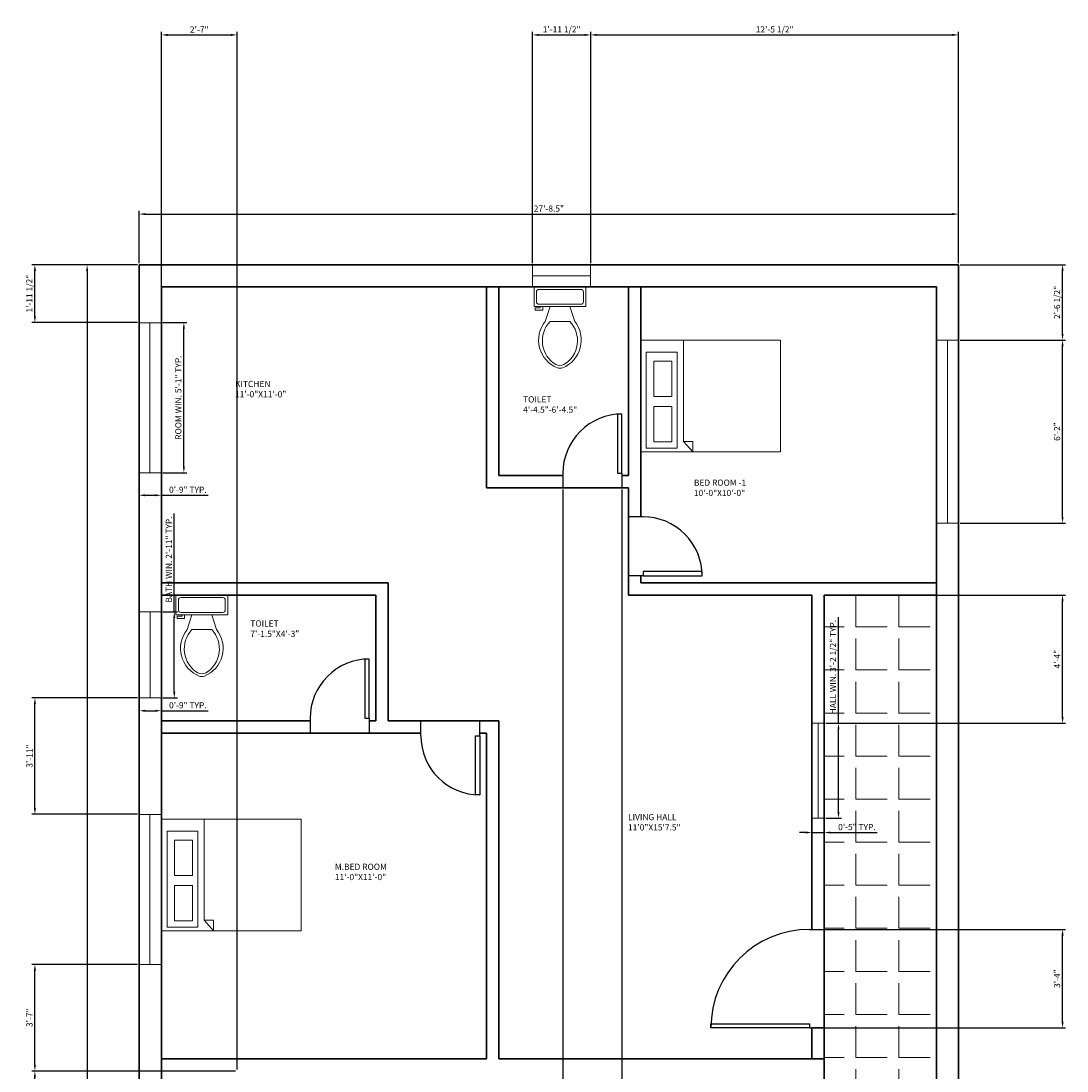
# Model space of a CAD drawing. Units: inches. Extents: x 4673 to 5097, y 7020 to 7947.
# Tile 3 of 3: x 4673 to 5097, y 7521 to 7947. Entities that reach past the tile are written whole.
import ezdxf

# ---------------------------------------------------------------- set-up
doc = ezdxf.new("R2010")
doc.units = ezdxf.units.IN
for name, color, linetype, lineweight in [('A-ANNO-DIMS', 244, 'Continuous', 18), ('A-AREA-IDEN', 7, 'Continuous', 18), ('A-DOOR', 4, 'Continuous', 25), ('A-FLOR-FIXT', 8, 'Continuous', 18), ('A-FLOR-PATT', 9, 'Continuous', 13), ('A-FURN', 152, 'Continuous', 18), ('A-GLAZ', 152, 'Continuous', 18), ('A-WALL', 7, 'Continuous', 35)]:
    doc.layers.add(name, color=color, linetype=linetype, lineweight=lineweight)
doc.styles.get("Standard").update_dxf_attribs({"font": 'arial.ttf'})
doc.dimstyles.new('ISO-25', dxfattribs={"dimtxt": 2.5, "dimasz": 2.5, "dimexe": 1.25, "dimexo": 0.625, "dimtad": 1, "dimlunit": 3, "dimtxsty": 'Standard', "dimcen": 2.5, "dimadec": 0, "dimazin": 0, "dimtfac": 1, "dimtmove": 0, "dimatfit": 3, "dimfxl": 1, "dimarcsym": 0})

# ---------------------------------------------------------------- blocks, each defined once
blk = doc.blocks.new('*U5')
for p, q in [((0, 0), (0, 6)), ((24, 0), (24, 6))]:
    blk.add_line(p, q)
blk.add_lwpolyline([(0, 0), (0, -24), (1.75, -24), (1.75, 0)], close=True)
blk.add_arc((0, 0), 24, 270, 0)
blk = doc.blocks.new('*U3')
for p, q in [((0, 0), (0, -6)), ((40, 0), (40, -6))]:
    blk.add_line(p, q)
blk.add_lwpolyline([(0, 0), (0, 40), (1.75, 40), (1.75, 0)], close=True)
blk.add_arc((0, 0), 40, 0, 90)
blk = doc.blocks.new('*U4')
for p, q in [((0, 0), (0, -6)), ((24, 0), (24, -6))]:
    blk.add_line(p, q)
blk.add_lwpolyline([(0, 0), (0, 24), (1.75, 24), (1.75, 0)], close=True)
blk.add_arc((0, 0), 24, 0, 90)
blk = doc.blocks.new('*U8')
for p, q in [((9.5, -6), (9.5, -2)), ((-10, -8.5), (-8, -8.5)), ((-10, -9.5), (-10, -8.5)), ((-8, -8.5), (-8, -8)), ((-7, -8), (-7, -9.5)), ((-4, -8), (-6, -14)), ((4, -8), (6, -14)), ((-7, -9.5), (-10, -9.5)), ((4, -14), (-4, -14))]:
    blk.add_line(p, q)
blk.add_lwpolyline([(10.5, -8), (10.5, 0), (-10.5, 0), (-10.5, -8)], close=True)
for points in [[(-9.5, -2), (-9.5, -6)], [(8.5, -1), (-8.5, -1)], [(-8.5, -7), (8.5, -7)]]:
    blk.add_lwpolyline(points)
for centre, radius, start, end in [((-8.62, -1.88), 0.884, 81.8699, 188.1301), ((8.62, -1.88), 0.884, 351.8699, 98.1301), ((-8.62, -6.12), 0.884, 171.8699, 278.1301), ((8.62, -6.12), 0.884, 261.8699, 8.1301), ((3.52, -21.58), 12.17, 141.4691, 247.9714), ((4.2, -21.82), 11.33, 136.3677, 238.9468), ((-3.52, -21.58), 12.17, 292.0284, 38.5307), ((-4.2, -21.82), 11.33, 301.053, 43.6321), ((0, -27.88), 4, 245.7318, 294.2682), ((0, -29), 4, 254.8605, 285.1395)]:
    blk.add_arc(centre, radius, start, end)
blk = doc.blocks.new('*D9')
at = {"layer": 'A-ANNO-DIMS', "color": 0, "lineweight": -2, "transparency": 16777216}
for p, q in [((4720.89, 7848.49), (4720.89, 7869.66)), ((4723.39, 7868.41), (5050.89, 7868.41)), ((5053.39, 7848.49), (5053.39, 7869.66))]:
    blk.add_line(p, q, dxfattribs=at)
at = {"layer": 'A-ANNO-DIMS', "color": 0, "transparency": 16777216}
for points in [[(4723.39, 7868.83), (4723.39, 7868), (4720.89, 7868.41)], [(5050.89, 7868.83), (5050.89, 7868), (5053.39, 7868.41)]]:
    blk.add_solid(points, dxfattribs=at)
at = {"layer": 'Defpoints', "color": 0, "transparency": 16777216}
for p in [(5053.39, 7868.41), (4720.89, 7847.86), (5053.39, 7847.86)]:
    blk.add_point(p, dxfattribs=at)
at = {"layer": 'A-ANNO-DIMS', "color": 0, "transparency": 16777216, "insert": (4887.14, 7870.32), "char_height": 2.5, "attachment_point": 5}
blk.add_mtext('27\'-8.5"', dxfattribs=at)
blk = doc.blocks.new('*D10')
at = {"layer": 'A-ANNO-DIMS', "color": 0, "lineweight": -2, "transparency": 16777216}
for p, q in [((4720.26, 7847.86), (4698.51, 7847.86)), ((4699.76, 7845.36), (4699.76, 7117.36)), ((4720.26, 7114.86), (4698.51, 7114.86))]:
    blk.add_line(p, q, dxfattribs=at)
at = {"layer": 'A-ANNO-DIMS', "color": 0, "transparency": 16777216}
for points in [[(4699.34, 7845.36), (4700.18, 7845.36), (4699.76, 7847.86)], [(4699.34, 7117.36), (4700.18, 7117.36), (4699.76, 7114.86)]]:
    blk.add_solid(points, dxfattribs=at)
at = {"layer": 'Defpoints', "color": 0, "transparency": 16777216}
for p in [(4720.89, 7847.86), (4699.76, 7114.86), (4720.89, 7114.86)]:
    blk.add_point(p, dxfattribs=at)
at = {"layer": 'A-ANNO-DIMS', "color": 0, "transparency": 16777216, "insert": (4697.86, 7481.36), "char_height": 2.5, "attachment_point": 5, "rotation": 90}
blk.add_mtext('61\'-1"', dxfattribs=at)
blk = doc.blocks.new('BED-DOUBLE')
for p, q in [((17.35, 45.28), (17.35, 4.23)), ((17.35, 4.23), (21.14, 0)), ((17.35, 4.23), (21.14, 4.23)), ((21.14, 0), (21.14, 4.23))]:
    blk.add_line(p, q)
for points in [[(0, 0), (0, 45.28), (56.77, 45.28), (56.77, 0)], [(2.29, 1.5), (2.29, 40.39), (14.79, 40.39), (14.79, 1.5)], [(5.28, 22.37), (5.28, 36.69), (12.64, 36.69), (12.64, 22.37)], [(5.28, 4.03), (5.28, 18.35), (12.64, 18.35), (12.64, 4.03)]]:
    blk.add_lwpolyline(points, close=True)
blk = doc.blocks.new('WIN-61IN')
for p, q in [((9, 60.82), (0, 60.82)), ((0.12, 60.89), (0.12, 0.07)), ((9, 60.82), (4.5, 60.82)), ((4.5, 60.82), (4.5, 0)), ((9.12, 0), (9.12, 60.82)), ((0, 0), (9, 0))]:
    blk.add_line(p, q)
blk = doc.blocks.new('WIN-HALL-38IN')
for p, q in [((5, 38.52), (0, 38.52)), ((0, 38.52), (0, 0)), ((5, 38.52), (2.5, 38.52)), ((2.5, 38.52), (2.5, 0)), ((5, 0), (5, 38.52)), ((0, 0), (5, 0))]:
    blk.add_line(p, q)
blk = doc.blocks.new('WIN-BATH-35IN')
for p, q in [((9, 34.94), (0, 34.94)), ((0, 34.94), (0, 0)), ((9, 34.94), (4.5, 34.94)), ((4.5, 34.94), (4.5, 0)), ((9, 0), (9, 34.94)), ((0, 0), (9, 0))]:
    blk.add_line(p, q)
blk = doc.blocks.new('*D17')
at = {"layer": 'A-ANNO-DIMS', "color": 0, "lineweight": -2, "transparency": 16777216}
for p, q in [((4730.51, 7824.39), (4740.27, 7824.39)), ((4739.02, 7766), (4739.02, 7821.89)), ((4730.51, 7763.5), (4740.27, 7763.5))]:
    blk.add_line(p, q, dxfattribs=at)
at = {"layer": 'A-ANNO-DIMS', "color": 0, "transparency": 16777216}
for points in [[(4738.6, 7821.89), (4739.44, 7821.89), (4739.02, 7824.39)], [(4738.6, 7766), (4739.44, 7766), (4739.02, 7763.5)]]:
    blk.add_solid(points, dxfattribs=at)
at = {"layer": 'Defpoints', "color": 0, "transparency": 16777216}
for p in [(4729.89, 7824.39), (4739.02, 7824.39), (4729.89, 7763.5)]:
    blk.add_point(p, dxfattribs=at)
at = {"layer": 'A-ANNO-DIMS', "color": 0, "transparency": 16777216, "insert": (4737.1, 7793.94), "char_height": 2.5, "attachment_point": 5, "rotation": 90}
blk.add_mtext('ROOM WIN. 5\'-1" TYP.', dxfattribs=at)
blk = doc.blocks.new('*D18')
at = {"layer": 'A-ANNO-DIMS', "color": 0, "lineweight": -2, "transparency": 16777216}
for p, q in [((4720.77, 7762.88), (4720.77, 7753.12)), ((4729.89, 7762.88), (4729.89, 7753.12)), ((4723.27, 7754.37), (4727.39, 7754.37)), ((4729.89, 7754.37), (4748.88, 7754.37))]:
    blk.add_line(p, q, dxfattribs=at)
at = {"layer": 'A-ANNO-DIMS', "color": 0, "transparency": 16777216}
for points in [[(4723.27, 7754.78), (4723.27, 7753.95), (4720.77, 7754.37)], [(4727.39, 7754.78), (4727.39, 7753.95), (4729.89, 7754.37)]]:
    blk.add_solid(points, dxfattribs=at)
at = {"layer": 'Defpoints', "color": 0, "transparency": 16777216}
for p in [(4720.77, 7763.5), (4729.89, 7763.5), (4729.89, 7754.37)]:
    blk.add_point(p, dxfattribs=at)
at = {"layer": 'A-ANNO-DIMS', "color": 0, "transparency": 16777216, "insert": (4740.63, 7756.27), "char_height": 2.5, "attachment_point": 5}
blk.add_mtext('0\'-9" TYP.', dxfattribs=at)
blk = doc.blocks.new('*D19')
at = {"layer": 'A-ANNO-DIMS', "color": 0, "lineweight": -2, "transparency": 16777216}
for p, q in [((4735.13, 7707.15), (4735.13, 7746.98)), ((4730.51, 7707.15), (4736.38, 7707.15)), ((4735.13, 7674.7), (4735.13, 7704.65)), ((4730.51, 7672.2), (4736.38, 7672.2))]:
    blk.add_line(p, q, dxfattribs=at)
at = {"layer": 'A-ANNO-DIMS', "color": 0, "transparency": 16777216}
for points in [[(4734.71, 7704.65), (4735.55, 7704.65), (4735.13, 7707.15)], [(4734.71, 7674.7), (4735.55, 7674.7), (4735.13, 7672.2)]]:
    blk.add_solid(points, dxfattribs=at)
at = {"layer": 'Defpoints', "color": 0, "transparency": 16777216}
for p in [(4729.89, 7707.15), (4735.13, 7707.15), (4729.89, 7672.2)]:
    blk.add_point(p, dxfattribs=at)
at = {"layer": 'A-ANNO-DIMS', "color": 0, "transparency": 16777216, "insert": (4733.25, 7728.31), "char_height": 2.5, "attachment_point": 5, "rotation": 90}
blk.add_mtext('BATH WIN. 2\'-11" TYP.', dxfattribs=at)
blk = doc.blocks.new('*D20')
at = {"layer": 'A-ANNO-DIMS', "color": 0, "lineweight": -2, "transparency": 16777216}
for p, q in [((4720.89, 7671.58), (4720.89, 7665.71)), ((4729.89, 7671.58), (4729.89, 7665.71)), ((4723.39, 7666.96), (4727.39, 7666.96)), ((4729.89, 7666.96), (4748.88, 7666.96))]:
    blk.add_line(p, q, dxfattribs=at)
at = {"layer": 'A-ANNO-DIMS', "color": 0, "transparency": 16777216}
for points in [[(4723.39, 7667.38), (4723.39, 7666.54), (4720.89, 7666.96)], [(4727.39, 7667.38), (4727.39, 7666.54), (4729.89, 7666.96)]]:
    blk.add_solid(points, dxfattribs=at)
at = {"layer": 'Defpoints', "color": 0, "transparency": 16777216}
for p in [(4720.89, 7672.2), (4729.89, 7672.2), (4729.89, 7666.96)]:
    blk.add_point(p, dxfattribs=at)
at = {"layer": 'A-ANNO-DIMS', "color": 0, "transparency": 16777216, "insert": (4740.63, 7668.86), "char_height": 2.5, "attachment_point": 5}
blk.add_mtext('0\'-9" TYP.', dxfattribs=at)
blk = doc.blocks.new('*D21')
at = {"layer": 'A-ANNO-DIMS', "color": 0, "lineweight": -2, "transparency": 16777216}
for p, q in [((5004.67, 7661.88), (5004.67, 7704.99)), ((4999.51, 7661.88), (5005.92, 7661.88)), ((5004.67, 7625.86), (5004.67, 7659.38)), ((4999.51, 7623.36), (5005.92, 7623.36))]:
    blk.add_line(p, q, dxfattribs=at)
at = {"layer": 'A-ANNO-DIMS', "color": 0, "transparency": 16777216}
for points in [[(5004.25, 7659.38), (5005.08, 7659.38), (5004.67, 7661.88)], [(5004.25, 7625.86), (5005.08, 7625.86), (5004.67, 7623.36)]]:
    blk.add_solid(points, dxfattribs=at)
at = {"layer": 'Defpoints', "color": 0, "transparency": 16777216}
for p in [(4998.89, 7661.88), (5004.67, 7661.88), (4998.89, 7623.36)]:
    blk.add_point(p, dxfattribs=at)
at = {"layer": 'A-ANNO-DIMS', "color": 0, "transparency": 16777216, "insert": (5002.75, 7684.68), "char_height": 2.5, "attachment_point": 5, "rotation": 90}
blk.add_mtext('HALL WIN. 3\'-2 1/2" TYP.', dxfattribs=at)
blk = doc.blocks.new('*D22')
at = {"layer": 'A-ANNO-DIMS', "color": 0, "lineweight": -2, "transparency": 16777216}
for p, q in [((4993.89, 7622.73), (4993.89, 7616.33)), ((4998.89, 7622.73), (4998.89, 7616.33)), ((4991.39, 7617.58), (4988.89, 7617.58)), ((4993.89, 7617.58), (4998.89, 7617.58)), ((5001.39, 7617.58), (5020.38, 7617.58))]:
    blk.add_line(p, q, dxfattribs=at)
at = {"layer": 'A-ANNO-DIMS', "color": 0, "transparency": 16777216}
for points in [[(4991.39, 7617.99), (4991.39, 7617.16), (4993.89, 7617.58)], [(5001.39, 7617.99), (5001.39, 7617.16), (4998.89, 7617.58)]]:
    blk.add_solid(points, dxfattribs=at)
at = {"layer": 'Defpoints', "color": 0, "transparency": 16777216}
for p in [(4993.89, 7623.36), (4998.89, 7623.36), (4998.89, 7617.58)]:
    blk.add_point(p, dxfattribs=at)
at = {"layer": 'A-ANNO-DIMS', "color": 0, "transparency": 16777216, "insert": (5012.13, 7619.48), "char_height": 2.5, "attachment_point": 5}
blk.add_mtext('0\'-5" TYP.', dxfattribs=at)
blk = doc.blocks.new('*D25')
at = {"layer": 'A-ANNO-DIMS', "color": 0, "lineweight": -2, "transparency": 16777216}
for p, q in [((5054.01, 7817.28), (5096.84, 7817.28)), ((5095.59, 7745.59), (5095.59, 7814.78)), ((5054.01, 7743.09), (5096.84, 7743.09))]:
    blk.add_line(p, q, dxfattribs=at)
at = {"layer": 'A-ANNO-DIMS', "color": 0, "transparency": 16777216}
for points in [[(5095.17, 7814.78), (5096.01, 7814.78), (5095.59, 7817.28)], [(5095.17, 7745.59), (5096.01, 7745.59), (5095.59, 7743.09)]]:
    blk.add_solid(points, dxfattribs=at)
at = {"layer": 'Defpoints', "color": 0, "transparency": 16777216}
for p in [(5053.39, 7817.28), (5095.59, 7817.28), (5053.39, 7743.09)]:
    blk.add_point(p, dxfattribs=at)
at = {"layer": 'A-ANNO-DIMS', "color": 0, "transparency": 16777216, "insert": (5093.69, 7780.18), "char_height": 2.5, "attachment_point": 5, "rotation": 90}
blk.add_mtext('6\'-2"', dxfattribs=at)
blk = doc.blocks.new('*D26')
at = {"layer": 'A-ANNO-DIMS', "color": 0, "lineweight": -2, "transparency": 16777216}
for p, q in [((5054.01, 7847.86), (5096.84, 7847.86)), ((5095.59, 7819.78), (5095.59, 7845.36)), ((5054.01, 7817.28), (5096.84, 7817.28))]:
    blk.add_line(p, q, dxfattribs=at)
at = {"layer": 'A-ANNO-DIMS', "color": 0, "transparency": 16777216}
for points in [[(5095.17, 7845.36), (5096.01, 7845.36), (5095.59, 7847.86)], [(5095.17, 7819.78), (5096.01, 7819.78), (5095.59, 7817.28)]]:
    blk.add_solid(points, dxfattribs=at)
at = {"layer": 'Defpoints', "color": 0, "transparency": 16777216}
for p in [(5053.39, 7847.86), (5095.59, 7847.86), (5053.39, 7817.28)]:
    blk.add_point(p, dxfattribs=at)
at = {"layer": 'A-ANNO-DIMS', "color": 0, "transparency": 16777216, "insert": (5093.67, 7832.57), "char_height": 2.5, "attachment_point": 5, "rotation": 90}
blk.add_mtext('2\'-6 1/2"', dxfattribs=at)
blk = doc.blocks.new('*D27')
at = {"layer": 'A-ANNO-DIMS', "color": 0, "lineweight": -2, "transparency": 16777216}
for p, q in [((4880.5, 7848.49), (4880.5, 7942.32)), ((4904.1, 7848.49), (4904.1, 7942.32)), ((4883, 7941.07), (4901.6, 7941.07))]:
    blk.add_line(p, q, dxfattribs=at)
at = {"layer": 'A-ANNO-DIMS', "color": 0, "transparency": 16777216}
for points in [[(4883, 7941.49), (4883, 7940.65), (4880.5, 7941.07)], [(4901.6, 7941.49), (4901.6, 7940.65), (4904.1, 7941.07)]]:
    blk.add_solid(points, dxfattribs=at)
at = {"layer": 'Defpoints', "color": 0, "transparency": 16777216}
for p in [(4904.1, 7941.07), (4880.5, 7847.86), (4904.1, 7847.86)]:
    blk.add_point(p, dxfattribs=at)
at = {"layer": 'A-ANNO-DIMS', "color": 0, "transparency": 16777216, "insert": (4892.3, 7942.99), "char_height": 2.5, "attachment_point": 5}
blk.add_mtext('1\'-11 1/2"', dxfattribs=at)
blk = doc.blocks.new('*D28')
at = {"layer": 'A-ANNO-DIMS', "color": 0, "lineweight": -2, "transparency": 16777216}
for p, q in [((4904.1, 7848.49), (4904.1, 7942.32)), ((5053.39, 7848.49), (5053.39, 7942.32)), ((4906.6, 7941.07), (5050.89, 7941.07))]:
    blk.add_line(p, q, dxfattribs=at)
at = {"layer": 'A-ANNO-DIMS', "color": 0, "transparency": 16777216}
for points in [[(4906.6, 7941.49), (4906.6, 7940.65), (4904.1, 7941.07)], [(5050.89, 7941.49), (5050.89, 7940.65), (5053.39, 7941.07)]]:
    blk.add_solid(points, dxfattribs=at)
at = {"layer": 'Defpoints', "color": 0, "transparency": 16777216}
for p in [(5053.39, 7941.07), (4904.1, 7847.86), (5053.39, 7847.86)]:
    blk.add_point(p, dxfattribs=at)
at = {"layer": 'A-ANNO-DIMS', "color": 0, "transparency": 16777216, "insert": (4978.74, 7942.99), "char_height": 2.5, "attachment_point": 5}
blk.add_mtext('12\'-5 1/2"', dxfattribs=at)
blk = doc.blocks.new('*D31')
at = {"layer": 'A-ANNO-DIMS', "color": 0, "lineweight": -2, "transparency": 16777216}
for p, q in [((4729.89, 7521.49), (4729.89, 7942.32)), ((4760.64, 7521.49), (4760.64, 7942.32)), ((4732.39, 7941.07), (4758.14, 7941.07))]:
    blk.add_line(p, q, dxfattribs=at)
at = {"layer": 'A-ANNO-DIMS', "color": 0, "transparency": 16777216}
for points in [[(4732.39, 7941.49), (4732.39, 7940.65), (4729.89, 7941.07)], [(4758.14, 7941.49), (4758.14, 7940.65), (4760.64, 7941.07)]]:
    blk.add_solid(points, dxfattribs=at)
at = {"layer": 'Defpoints', "color": 0, "transparency": 16777216}
for p in [(4760.64, 7941.07), (4729.89, 7520.86), (4760.64, 7520.86)]:
    blk.add_point(p, dxfattribs=at)
at = {"layer": 'A-ANNO-DIMS', "color": 0, "transparency": 16777216, "insert": (4745.26, 7942.95), "char_height": 2.5, "attachment_point": 5}
blk.add_mtext('2\'-7"', dxfattribs=at)
blk = doc.blocks.new('*D32')
at = {"layer": 'A-ANNO-DIMS', "color": 0, "lineweight": -2, "transparency": 16777216}
for p, q in [((4760.01, 7520.86), (4677.32, 7520.86)), ((4678.57, 7493.36), (4678.57, 7518.36)), ((4760.01, 7490.86), (4677.32, 7490.86))]:
    blk.add_line(p, q, dxfattribs=at)
at = {"layer": 'A-ANNO-DIMS', "color": 0, "transparency": 16777216}
for points in [[(4678.15, 7518.36), (4678.99, 7518.36), (4678.57, 7520.86)], [(4678.15, 7493.36), (4678.99, 7493.36), (4678.57, 7490.86)]]:
    blk.add_solid(points, dxfattribs=at)
at = {"layer": 'Defpoints', "color": 0, "transparency": 16777216}
for p in [(4678.57, 7520.86), (4760.64, 7520.86), (4760.64, 7490.86)]:
    blk.add_point(p, dxfattribs=at)
at = {"layer": 'A-ANNO-DIMS', "color": 0, "transparency": 16777216, "insert": (4676.67, 7505.86), "char_height": 2.5, "attachment_point": 5, "rotation": 90}
blk.add_mtext('2\'-6"', dxfattribs=at)
blk = doc.blocks.new('*D34')
at = {"layer": 'A-ANNO-DIMS', "color": 0, "lineweight": -2, "transparency": 16777216}
for p, q in [((4994.51, 7578.31), (5096.84, 7578.31)), ((5095.59, 7540.82), (5095.59, 7575.81)), ((4994.51, 7538.32), (5096.84, 7538.32))]:
    blk.add_line(p, q, dxfattribs=at)
at = {"layer": 'A-ANNO-DIMS', "color": 0, "transparency": 16777216}
for points in [[(5095.17, 7575.81), (5096.01, 7575.81), (5095.59, 7578.31)], [(5095.17, 7540.82), (5096.01, 7540.82), (5095.59, 7538.32)]]:
    blk.add_solid(points, dxfattribs=at)
at = {"layer": 'Defpoints', "color": 0, "transparency": 16777216}
for p in [(4993.89, 7578.31), (5095.59, 7578.31), (4993.89, 7538.32)]:
    blk.add_point(p, dxfattribs=at)
at = {"layer": 'A-ANNO-DIMS', "color": 0, "transparency": 16777216, "insert": (5093.69, 7558.31), "char_height": 2.5, "attachment_point": 5, "rotation": 90}
blk.add_mtext('3\'-4"', dxfattribs=at)
blk = doc.blocks.new('*D35')
at = {"layer": 'A-ANNO-DIMS', "color": 0, "lineweight": -2, "transparency": 16777216}
for p, q in [((4892.8, 7756.68), (4892.8, 7020.41)), ((4916.8, 7756.68), (4916.8, 7020.41)), ((4895.3, 7021.66), (4914.3, 7021.66))]:
    blk.add_line(p, q, dxfattribs=at)
at = {"layer": 'A-ANNO-DIMS', "color": 0, "transparency": 16777216}
for points in [[(4895.3, 7022.08), (4895.3, 7021.25), (4892.8, 7021.66)], [(4914.3, 7022.08), (4914.3, 7021.25), (4916.8, 7021.66)]]:
    blk.add_solid(points, dxfattribs=at)
at = {"layer": 'Defpoints', "color": 0, "transparency": 16777216}
for p in [(4892.8, 7757.31), (4916.8, 7757.31), (4916.8, 7021.66)]:
    blk.add_point(p, dxfattribs=at)
at = {"layer": 'A-ANNO-DIMS', "color": 0, "transparency": 16777216, "insert": (4904.8, 7023.56), "char_height": 2.5, "attachment_point": 5}
blk.add_mtext('2\'-0"', dxfattribs=at)
blk = doc.blocks.new('*D40')
at = {"layer": 'A-ANNO-DIMS', "color": 0, "lineweight": -2, "transparency": 16777216}
for p, q in [((4720.14, 7564.08), (4677.32, 7564.08)), ((4678.57, 7523.36), (4678.57, 7561.58)), ((4729.26, 7520.86), (4677.32, 7520.86))]:
    blk.add_line(p, q, dxfattribs=at)
at = {"layer": 'A-ANNO-DIMS', "color": 0, "transparency": 16777216}
for points in [[(4678.15, 7561.58), (4678.99, 7561.58), (4678.57, 7564.08)], [(4678.15, 7523.36), (4678.99, 7523.36), (4678.57, 7520.86)]]:
    blk.add_solid(points, dxfattribs=at)
at = {"layer": 'Defpoints', "color": 0, "transparency": 16777216}
for p in [(4678.57, 7564.08), (4720.77, 7564.08), (4729.89, 7520.86)]:
    blk.add_point(p, dxfattribs=at)
at = {"layer": 'A-ANNO-DIMS', "color": 0, "transparency": 16777216, "insert": (4676.67, 7542.47), "char_height": 2.5, "attachment_point": 5, "rotation": 90}
blk.add_mtext('3\'-7"', dxfattribs=at)
blk = doc.blocks.new('*D41')
at = {"layer": 'A-ANNO-DIMS', "color": 0, "lineweight": -2, "transparency": 16777216}
for p, q in [((4720.26, 7672.2), (4677.32, 7672.2)), ((4678.57, 7627.47), (4678.57, 7669.7)), ((4720.26, 7624.97), (4677.32, 7624.97))]:
    blk.add_line(p, q, dxfattribs=at)
at = {"layer": 'A-ANNO-DIMS', "color": 0, "transparency": 16777216}
for points in [[(4678.15, 7669.7), (4678.99, 7669.7), (4678.57, 7672.2)], [(4678.15, 7627.47), (4678.99, 7627.47), (4678.57, 7624.97)]]:
    blk.add_solid(points, dxfattribs=at)
at = {"layer": 'Defpoints', "color": 0, "transparency": 16777216}
for p in [(4678.57, 7672.2), (4720.89, 7672.2), (4720.89, 7624.97)]:
    blk.add_point(p, dxfattribs=at)
at = {"layer": 'A-ANNO-DIMS', "color": 0, "transparency": 16777216, "insert": (4676.67, 7648.59), "char_height": 2.5, "attachment_point": 5, "rotation": 90}
blk.add_mtext('3\'-11"', dxfattribs=at)
blk = doc.blocks.new('*D42')
at = {"layer": 'A-ANNO-DIMS', "color": 0, "lineweight": -2, "transparency": 16777216}
for p, q in [((4720.26, 7847.86), (4677.32, 7847.86)), ((4678.57, 7826.89), (4678.57, 7845.36)), ((4720.26, 7824.39), (4677.32, 7824.39))]:
    blk.add_line(p, q, dxfattribs=at)
at = {"layer": 'A-ANNO-DIMS', "color": 0, "transparency": 16777216}
for points in [[(4678.15, 7845.36), (4678.99, 7845.36), (4678.57, 7847.86)], [(4678.15, 7826.89), (4678.99, 7826.89), (4678.57, 7824.39)]]:
    blk.add_solid(points, dxfattribs=at)
at = {"layer": 'Defpoints', "color": 0, "transparency": 16777216}
for p in [(4678.57, 7847.86), (4720.89, 7847.86), (4720.89, 7824.39)]:
    blk.add_point(p, dxfattribs=at)
at = {"layer": 'A-ANNO-DIMS', "color": 0, "transparency": 16777216, "insert": (4676.65, 7836.12), "char_height": 2.5, "attachment_point": 5, "rotation": 90}
blk.add_mtext('1\'-11 1/2"', dxfattribs=at)
blk = doc.blocks.new('*D46')
at = {"layer": 'A-ANNO-DIMS', "color": 0, "lineweight": -2, "transparency": 16777216}
for p, q in [((4999.51, 7713.86), (5096.84, 7713.86)), ((5095.59, 7664.38), (5095.59, 7711.36)), ((4999.51, 7661.88), (5096.84, 7661.88))]:
    blk.add_line(p, q, dxfattribs=at)
at = {"layer": 'A-ANNO-DIMS', "color": 0, "transparency": 16777216}
for points in [[(5095.17, 7711.36), (5096.01, 7711.36), (5095.59, 7713.86)], [(5095.17, 7664.38), (5096.01, 7664.38), (5095.59, 7661.88)]]:
    blk.add_solid(points, dxfattribs=at)
at = {"layer": 'Defpoints', "color": 0, "transparency": 16777216}
for p in [(4998.89, 7713.86), (5095.59, 7713.86), (4998.89, 7661.88)]:
    blk.add_point(p, dxfattribs=at)
at = {"layer": 'A-ANNO-DIMS', "color": 0, "transparency": 16777216, "insert": (5093.71, 7687.87), "char_height": 2.5, "attachment_point": 5, "rotation": 90}
blk.add_mtext('4\'-4"', dxfattribs=at)

msp = doc.modelspace()

# ---------------------------------------------------------------- hatches: boundary and pattern name
at = {"layer": 'A-FLOR-PATT'}
h = msp.add_hatch(dxfattribs=at)
h.set_pattern_fill('ANGLE', color=256, scale=2.5)
h.set_pattern_definition([(0, (0, 0), (0, 17.4625), [12.7, -4.7625]), (90, (0, 0), (-17.4625, 1e-15), [12.7, -4.7625])])
h.paths.add_polyline_path([(5044.389, 7713.863), (4998.889, 7713.863), (4998.889, 7243.863), (5044.389, 7243.863)])

# ---------------------------------------------------------------- linework, layer by layer
at = {"layer": 'A-GLAZ'}
for p, q in [((4880.5, 7847.863), (4880.5, 7838.863)), ((4904.097, 7847.863), (4880.5, 7847.863)), ((4880.5, 7847.863), (4880.5, 7843.363)), ((4904.097, 7838.863), (4904.097, 7847.863)), ((4880.5, 7843.363), (4904.097, 7843.363)), ((4880.5, 7838.863), (4904.097, 7838.863)), ((5044.389, 7817.278), (5053.389, 7817.278)), ((5044.389, 7743.09), (5044.389, 7817.278)), ((5044.389, 7817.278), (5048.889, 7817.278)), ((5048.889, 7817.278), (5048.889, 7743.09)), ((5053.389, 7817.278), (5053.389, 7743.09)), ((5053.389, 7743.09), (5044.389, 7743.09))]:
    msp.add_line(p, q, dxfattribs=at)
at = {"layer": 'A-WALL'}
for p, q in [((4720.889, 7847.863), (4720.889, 7114.863)), ((4720.889, 7847.863), (5053.389, 7847.863)), ((5053.389, 7847.863), (5053.389, 7293.326)), ((4729.889, 7838.863), (4729.889, 7718.863)), ((4729.889, 7838.863), (4861.889, 7838.863)), ((4861.889, 7838.863), (4861.889, 7757.363)), ((4861.889, 7838.863), (4861.889, 7757.363)), ((4861.889, 7838.863), (4919.389, 7838.863)), ((4866.889, 7838.863), (4866.889, 7762.363)), ((4866.889, 7838.863), (4866.889, 7762.363)), ((4919.389, 7838.863), (4919.389, 7762.363)), ((4919.389, 7838.863), (5044.389, 7838.863)), ((4924.389, 7838.863), (4924.389, 7745.64)), ((5044.389, 7838.863), (5044.389, 7713.863)), ((4866.889, 7762.363), (4892.804, 7762.363)), ((4916.804, 7762.363), (4919.389, 7762.363)), ((4861.889, 7757.363), (4919.389, 7757.363)), ((4919.389, 7757.363), (4919.389, 7713.863)), ((4924.389, 7721.64), (4924.389, 7718.863)), ((4729.889, 7718.863), (4821.889, 7718.863)), ((4729.889, 7718.863), (4821.889, 7718.863)), ((4729.889, 7718.863), (4729.889, 7662.863)), ((4821.889, 7718.863), (4821.889, 7662.863)), ((4924.389, 7718.863), (5044.389, 7718.863)), ((4924.389, 7718.863), (5044.389, 7718.863)), ((4729.889, 7713.863), (4816.889, 7713.863)), ((4816.889, 7713.863), (4816.889, 7662.863)), ((4993.889, 7713.821), (4919.389, 7713.821)), ((4993.889, 7713.821), (4993.889, 7582.7)), ((4998.889, 7713.863), (5044.389, 7713.863)), ((4998.889, 7713.863), (4998.889, 7243.863)), ((5044.389, 7713.863), (5044.389, 7238.863)), ((4729.889, 7662.863), (4790.262, 7662.863)), ((4729.889, 7662.863), (4729.889, 7525.863)), ((4814.262, 7662.863), (4816.889, 7662.863)), ((4821.889, 7662.863), (4866.889, 7662.863)), ((4866.889, 7662.863), (4866.889, 7525.863)), ((4729.889, 7657.863), (4835.175, 7657.863)), ((4859.175, 7657.863), (4861.889, 7657.863)), ((4861.889, 7657.863), (4861.889, 7525.863)), ((4993.889, 7582.7), (4993.889, 7578.307)), ((4993.889, 7538.322), (4998.889, 7538.322)), ((4998.889, 7538.322), (4993.889, 7538.322)), ((4993.889, 7538.322), (4993.889, 7525.863)), ((4998.889, 7525.863), (4998.889, 7538.322)), ((4729.889, 7525.863), (4861.889, 7525.863)), ((4729.889, 7525.863), (4729.889, 7443.863)), ((4866.889, 7525.863), (4998.889, 7525.863))]:
    msp.add_line(p, q, dxfattribs=at)

# ---------------------------------------------------------------- block references
at = {"layer": 'A-DOOR'}
for name, p, rotation in [('*U5', (4916.804, 7763.308), 180), ('*U5', (4925.365, 7721.64), 89.99999999999999), ('*U5', (4814.262, 7663.956), 180), ('*U4', (4859.175, 7656.853), 180), ('*U3', (4992.877, 7538.307), 90)]:
    msp.add_blockref(name, p, dxfattribs=dict(at, rotation=rotation))
at = {"layer": 'A-FLOR-FIXT'}
for p in [(4891.63, 7838.869), (4746.31, 7713.869)]:
    msp.add_blockref('*U8', p, dxfattribs=at)
at = {"layer": 'A-FURN'}
for p in [(4924.389, 7772.001), (4729.889, 7577.748)]:
    msp.add_blockref('BED-DOUBLE', p, dxfattribs=at)
at = {"layer": 'A-GLAZ'}
for name, p in [('WIN-61IN', (4720.769, 7763.501)), ('WIN-BATH-35IN', (4720.889, 7672.203)), ('WIN-HALL-38IN', (4993.889, 7623.355)), ('WIN-61IN', (4720.769, 7564.082))]:
    msp.add_blockref(name, p, dxfattribs=at)

# ---------------------------------------------------------------- texts
at = {"layer": 'A-AREA-IDEN', "char_height": 2.5, "attachment_point": 1}
for s, width, insert in [('{KITCHEN\\P11\'-0"X11\'-0"}', 86.95948, (4759.784, 7800.765)), ('TOILET\\P4\'-4.5"-6\'-4.5"', 19.88915, (4876.694, 7794.504)), ('BED ROOM -1\\P10\'-0"X10\'-0"', 68.60052, (4945.982, 7760.725)), ('TOILET\\P7\'-1.5"X4\'-3"', 28.47558, (4766, 7703.602)), ('LIVING HALL\\P11\'0"X15\'7.5"', 50.37915, (4919.268, 7625.093)), ('M.BED ROOM\\P11\'-0"X11\'-0"', 33.54132, (4800.309, 7604.943))]:
    msp.add_mtext_dynamic_manual_height_columns(s, width=width, gutter_width=12.5, heights=[0], dxfattribs=dict(at, insert=insert))

# ---------------------------------------------------------------- dimensions: what is measured, and where the dimension line sits
at = {"layer": 'A-ANNO-DIMS'}
for base, p1, p2, override, picture, middle in [((4904.097, 7941.069), (4880.5, 7847.863), (4904.097, 7847.863), {"dimdec": 1, "dimlfac": 1, "dimrnd": 0, "dimzin": 1, "dimdsep": 46, "dimlunit": 4, "dimfrac": 2}, '*D27', (4892.298, 7942.987)), ((5053.389, 7941.069), (4904.097, 7847.863), (5053.389, 7847.863), {"dimdec": 1, "dimlfac": 1, "dimrnd": 0, "dimzin": 1, "dimdsep": 46, "dimlunit": 4, "dimfrac": 2}, '*D28', (4978.743, 7942.987)), ((4760.6392, 7941.0691), (4729.8886, 7520.8629), (4760.6392, 7520.8629), {"dimdec": 1, "dimlfac": 1, "dimrnd": 0, "dimzin": 1, "dimdsep": 46, "dimlunit": 4, "dimfrac": 2}, '*D31', (4745.2639, 7942.9492)), ((5053.389, 7868.414), (4720.889, 7847.863), (5053.389, 7847.863), {"dimclrd": 0, "dimclre": 0, "dimclrt": 0}, '*D9', (4887.139, 7870.315)), ((4916.804, 7021.663), (4892.804, 7757.308), (4916.804, 7757.308), {"dimdec": 1, "dimlfac": 1, "dimrnd": 0, "dimzin": 1, "dimdsep": 46, "dimlunit": 4, "dimfrac": 2}, '*D35', (4904.804, 7023.564))]:
    dim = msp.add_linear_dim(base=base, p1=p1, p2=p2, dimstyle='ISO-25', override=override, dxfattribs=at)
    dim.commit()
    dim.dimension.update_dxf_attribs({"geometry": picture, "text_midpoint": middle})
for base, p1, p2, override, picture, middle in [((4678.569, 7847.863), (4720.889, 7824.387), (4720.889, 7847.863), {"dimdec": 1, "dimlfac": 1, "dimrnd": 0, "dimzin": 1, "dimdsep": 46, "dimlunit": 4, "dimfrac": 2}, '*D42', (4676.652, 7836.125)), ((4699.76, 7114.863), (4720.889, 7847.863), (4720.889, 7114.863), {"dimclrd": 0, "dimclre": 0, "dimclrt": 0}, '*D10', (4697.858, 7481.363)), ((5095.589, 7847.863), (5053.389, 7817.278), (5053.389, 7847.863), {"dimdec": 1, "dimlfac": 1, "dimrnd": 0, "dimzin": 1, "dimdsep": 46, "dimlunit": 4, "dimfrac": 2}, '*D26', (5093.671, 7832.57)), ((5095.589, 7817.278), (5053.389, 7743.09), (5053.389, 7817.278), {"dimdec": 1, "dimlfac": 1, "dimrnd": 0, "dimzin": 1, "dimdsep": 46, "dimlunit": 4, "dimfrac": 2}, '*D25', (5093.687, 7780.184)), ((5095.589, 7713.863), (4998.889, 7661.876), (4998.889, 7713.863), {"dimdec": 1, "dimlfac": 1, "dimrnd": 0, "dimzin": 1, "dimdsep": 46, "dimlunit": 4, "dimfrac": 2}, '*D46', (5093.714, 7687.869)), ((4678.569, 7672.202), (4720.889, 7624.968), (4720.889, 7672.202), {"dimdec": 1, "dimlfac": 1, "dimrnd": 0, "dimzin": 1, "dimdsep": 46, "dimlunit": 4, "dimfrac": 2}, '*D41', (4676.667, 7648.585)), ((5095.589, 7578.307), (4993.889, 7538.322), (4993.889, 7578.307), {"dimdec": 1, "dimlfac": 1, "dimrnd": 0, "dimzin": 1, "dimdsep": 46, "dimlunit": 4, "dimfrac": 2}, '*D34', (5093.686, 7558.315)), ((4678.569, 7564.082), (4729.889, 7520.863), (4720.769, 7564.082), {"dimdec": 1, "dimlfac": 1, "dimrnd": 0, "dimzin": 1, "dimdsep": 46, "dimlunit": 4, "dimfrac": 2}, '*D40', (4676.667, 7542.472)), ((4678.569, 7520.863), (4760.639, 7490.863), (4760.639, 7520.863), {"dimdec": 1, "dimlfac": 1, "dimrnd": 0, "dimzin": 1, "dimdsep": 46, "dimlunit": 4, "dimfrac": 2}, '*D32', (4676.668, 7505.863))]:
    dim = msp.add_linear_dim(base=base, p1=p1, p2=p2, angle=90, dimstyle='ISO-25', override=override, dxfattribs=at)
    dim.commit()
    dim.dimension.update_dxf_attribs({"geometry": picture, "text_midpoint": middle})
for base, p1, p2, text, picture, middle in [((4739.021, 7824.387), (4729.889, 7763.501), (4729.889, 7824.387), 'ROOM WIN. <> TYP.', '*D17', (4737.103, 7793.944)), ((4735.13, 7707.146), (4729.889, 7672.202), (4729.889, 7707.146), 'BATH WIN. <> TYP.', '*D19', (4733.249, 7728.313)), ((5004.667, 7661.876), (4998.889, 7623.355), (4998.889, 7661.876), 'HALL WIN. <> TYP.', '*D21', (5002.748, 7684.684))]:
    dim = msp.add_linear_dim(base=base, p1=p1, p2=p2, angle=90, text=text, dimstyle='ISO-25', override={"dimdec": 1, "dimlfac": 1, "dimrnd": 0, "dimzin": 1, "dimdsep": 46, "dimlunit": 4, "dimfrac": 2}, dxfattribs=at)
    dim.commit()
    dim.dimension.update_dxf_attribs({"geometry": picture, "text_midpoint": middle})
for base, p1, p2, picture, middle in [((4729.889, 7754.368), (4720.769, 7763.501), (4729.889, 7763.501), '*D18', (4740.633, 7756.27)), ((4729.889, 7666.961), (4720.889, 7672.202), (4729.889, 7672.202), '*D20', (4740.633, 7668.862)), ((4998.889, 7617.577), (4993.889, 7623.355), (4998.889, 7623.355), '*D22', (5012.133, 7619.479))]:
    dim = msp.add_linear_dim(base=base, p1=p1, p2=p2, text='<> TYP.', dimstyle='ISO-25', override={"dimdec": 1, "dimlfac": 1, "dimrnd": 0, "dimzin": 1, "dimdsep": 46, "dimlunit": 4, "dimfrac": 2}, dxfattribs=at)
    dim.commit()
    dim.dimension.update_dxf_attribs({"geometry": picture, "text_midpoint": middle})

doc.saveas('drawing.dxf')
